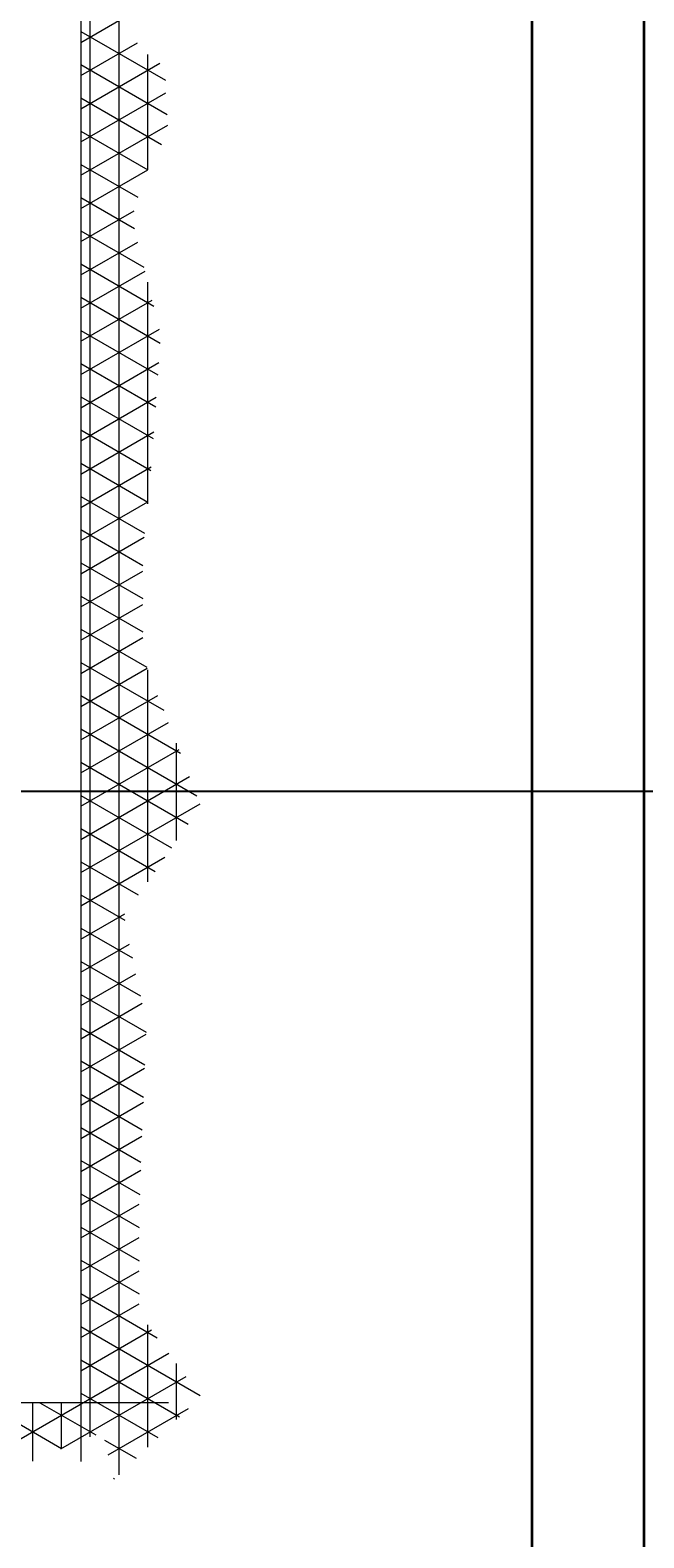
# Model space of a CAD drawing. Units: inches. Extents: x 3731 to 4318, y 1310 to 2388.
# Tile 54 of 57: x 4212 to 4239, y 2229 to 2296. Entities that reach past the tile are written whole.
import ezdxf

# ---------------------------------------------------------------- set-up
doc = ezdxf.new("R2010")
doc.units = ezdxf.units.IN
for name, color, linetype, lineweight in [('A-ANNO-DIMS', 2, 'Continuous', 18), ('A-FURN', 8, 'Continuous', 13), ('A-WALL', 7, 'Continuous', 35)]:
    doc.layers.add(name, color=color, linetype=linetype, lineweight=lineweight)
doc.styles.get("Standard").update_dxf_attribs({"font": 'arial.ttf'})
doc.dimstyles.get("Standard").update_dxf_attribs({"dimtxt": 0.18, "dimasz": 0.18, "dimexe": 0.18, "dimexo": 0.0625, "dimgap": 0.09, "dimtad": 0, "dimtih": 1, "dimtoh": 1, "dimdec": 4, "dimzin": 0, "dimdsep": 46, "dimtxsty": 'Standard', "dimcen": 0.09, "dimadec": 0, "dimazin": 0, "dimtfac": 1, "dimtdec": 4, "dimtofl": 0, "dimtmove": 0, "dimatfit": 3, "dimfxl": 1, "dimtolj": 1, "dimtzin": 0, "dimarcsym": 0})

# ---------------------------------------------------------------- blocks, each defined once
blk = doc.blocks.new('A$C200C7901')
for p, q in [((2.3121, 1.6596), (2.3121, 0.0201)), ((2.4073, 0.0839), (0.9625, 0.0839))]:
    blk.add_line(p, q)
at = {"linetype": 'ByBlock'}
for p, q in [((2.3224, 0.0468), (2.3224, 1.6627)), ((2.3224, 0.0468), (2.3224, 1.6627)), ((2.3537, 0.0056), (2.3537, 1.634)), ((2.3537, 0.0056), (2.3537, 1.634)), ((2.3121, 1.5619), (2.3654, 1.5926)), ((2.3121, 1.5619), (2.3654, 1.5926)), ((2.3121, 1.5738), (2.404, 1.5208)), ((2.3121, 1.5738), (2.404, 1.5208)), ((2.3121, 1.5258), (2.3739, 1.5615)), ((2.3121, 1.5258), (2.3739, 1.5615)), ((2.3849, 1.4236), (2.3849, 1.5486)), ((2.3849, 1.4236), (2.3849, 1.5486)), ((2.3121, 1.4897), (2.3979, 1.5393)), ((2.3121, 1.4897), (2.3979, 1.5393)), ((2.3121, 1.5377), (2.406, 1.4835)), ((2.3121, 1.5377), (2.406, 1.4835)), ((2.3121, 1.4537), (2.4047, 1.5071)), ((2.3121, 1.4537), (2.4047, 1.5071)), ((2.3121, 1.5016), (2.3997, 1.4511)), ((2.3121, 1.5016), (2.3997, 1.4511)), ((2.3121, 1.4176), (2.4067, 1.4721)), ((2.3121, 1.4176), (2.4067, 1.4721)), ((2.3121, 1.4655), (2.3849, 1.4235)), ((2.3121, 1.4655), (2.3849, 1.4235)), ((2.3121, 1.4294), (2.3741, 1.3937)), ((2.3121, 1.4294), (2.3741, 1.3937)), ((2.3121, 1.3815), (2.3848, 1.4235)), ((2.3121, 1.3815), (2.3848, 1.4235)), ((2.3121, 1.3934), (2.3703, 1.3598)), ((2.3121, 1.3934), (2.3703, 1.3598)), ((2.3121, 1.3454), (2.37, 1.3788)), ((2.3121, 1.3454), (2.37, 1.3788)), ((2.3121, 1.3573), (2.3808, 1.3176)), ((2.3121, 1.3573), (2.3808, 1.3176)), ((2.3121, 1.3093), (2.374, 1.345)), ((2.3121, 1.3093), (2.374, 1.345)), ((2.3121, 1.3212), (2.3914, 1.2754)), ((2.3121, 1.3212), (2.3914, 1.2754)), ((2.3121, 1.2732), (2.3819, 1.3135)), ((2.3121, 1.2732), (2.3819, 1.3135)), ((2.3849, 1.0607), (2.3849, 1.3013)), ((2.3849, 1.0607), (2.3849, 1.3013)), ((2.3121, 1.2851), (2.3985, 1.2352)), ((2.3121, 1.2851), (2.3985, 1.2352)), ((2.3121, 1.2371), (2.3898, 1.282)), ((2.3121, 1.2371), (2.3898, 1.282)), ((2.3121, 1.2011), (2.3976, 1.2504)), ((2.3121, 1.2011), (2.3976, 1.2504)), ((2.3121, 1.249), (2.396, 1.2006)), ((2.3121, 1.249), (2.396, 1.2006)), ((2.3121, 1.165), (2.397, 1.214)), ((2.3121, 1.165), (2.397, 1.214)), ((2.3121, 1.2129), (2.3935, 1.166)), ((2.3121, 1.2129), (2.3935, 1.166)), ((2.3121, 1.1768), (2.3909, 1.1314)), ((2.3121, 1.1768), (2.3909, 1.1314)), ((2.3121, 1.1289), (2.3942, 1.1763)), ((2.3121, 1.1289), (2.3942, 1.1763)), ((2.3121, 1.1408), (2.3884, 1.0967)), ((2.3121, 1.1408), (2.3884, 1.0967)), ((2.3121, 1.0928), (2.3915, 1.1386)), ((2.3121, 1.0928), (2.3915, 1.1386)), ((2.3121, 1.1047), (2.3851, 1.0625)), ((2.3121, 1.1047), (2.3851, 1.0625)), ((2.3121, 1.0567), (2.3887, 1.1009)), ((2.3121, 1.0567), (2.3887, 1.1009)), ((2.3121, 1.0686), (2.3813, 1.0286)), ((2.3121, 1.0686), (2.3813, 1.0286)), ((2.3121, 1.0206), (2.3851, 1.0628)), ((2.3121, 1.0206), (2.3851, 1.0628)), ((2.3121, 1.0325), (2.3795, 0.9936)), ((2.3121, 1.0325), (2.3795, 0.9936)), ((2.3121, 0.9846), (2.3809, 1.0242)), ((2.3121, 0.9846), (2.3809, 1.0242)), ((2.3121, 0.9964), (2.3795, 0.9575)), ((2.3121, 0.9964), (2.3795, 0.9575)), ((2.3121, 0.9485), (2.3795, 0.9874)), ((2.3121, 0.9485), (2.3795, 0.9874)), ((2.3121, 0.9603), (2.3795, 0.9215)), ((2.3121, 0.9603), (2.3795, 0.9215)), ((2.3121, 0.9124), (2.3795, 0.9513)), ((2.3121, 0.9124), (2.3795, 0.9513)), ((2.3121, 0.9243), (2.3838, 0.8829)), ((2.3121, 0.9243), (2.3838, 0.8829)), ((2.3121, 0.8763), (2.3795, 0.9152)), ((2.3121, 0.8763), (2.3795, 0.9152)), ((2.3121, 0.8882), (2.4022, 0.8362)), ((2.3121, 0.8882), (2.4022, 0.8362)), ((2.3121, 0.8402), (2.3842, 0.8818)), ((2.3121, 0.8402), (2.3842, 0.8818)), ((2.3849, 0.6497), (2.3849, 0.8801)), ((2.3849, 0.6497), (2.3849, 0.8801)), ((2.3121, 0.8041), (2.3958, 0.8524)), ((2.3121, 0.8041), (2.3958, 0.8524)), ((2.3121, 0.8521), (2.4205, 0.7895)), ((2.3121, 0.8521), (2.4205, 0.7895)), ((2.3121, 0.7681), (2.4073, 0.823)), ((2.3121, 0.7681), (2.4073, 0.823)), ((2.3121, 0.816), (2.4384, 0.7431)), ((2.3121, 0.816), (2.4384, 0.7431)), ((2.3121, 0.732), (2.4189, 0.7936)), ((2.3121, 0.732), (2.4189, 0.7936)), ((2.4162, 0.6946), (2.4162, 0.8006)), ((2.4162, 0.6946), (2.4162, 0.8006)), ((2.3121, 0.7799), (2.4287, 0.7126)), ((2.3121, 0.7799), (2.4287, 0.7126)), ((2.3121, 0.6959), (2.4303, 0.7641)), ((2.3121, 0.6959), (2.4303, 0.7641)), ((2.3121, 0.7438), (2.4108, 0.6869)), ((2.3121, 0.7438), (2.4108, 0.6869)), ((2.3121, 0.6598), (2.4417, 0.7346)), ((2.3121, 0.6598), (2.4417, 0.7346)), ((2.3121, 0.7078), (2.3929, 0.6611)), ((2.3121, 0.7078), (2.3929, 0.6611)), ((2.3121, 0.6237), (2.4036, 0.6765)), ((2.3121, 0.6237), (2.4036, 0.6765)), ((2.3121, 0.6717), (2.3744, 0.6357)), ((2.3121, 0.6717), (2.3744, 0.6357)), ((2.3121, 0.6356), (2.3598, 0.6081)), ((2.3121, 0.6356), (2.3598, 0.6081)), ((2.3121, 0.5876), (2.3598, 0.6151)), ((2.3121, 0.5876), (2.3598, 0.6151)), ((2.3121, 0.5995), (2.3682, 0.5671)), ((2.3121, 0.5995), (2.3682, 0.5671)), ((2.3121, 0.5515), (2.365, 0.5821)), ((2.3121, 0.5515), (2.365, 0.5821)), ((2.3121, 0.5634), (2.3771, 0.5259)), ((2.3121, 0.5634), (2.3771, 0.5259)), ((2.3121, 0.5155), (2.3719, 0.55)), ((2.3121, 0.5155), (2.3719, 0.55)), ((2.3121, 0.5273), (2.383, 0.4864)), ((2.3121, 0.5273), (2.383, 0.4864)), ((2.3121, 0.4794), (2.3788, 0.5179)), ((2.3121, 0.4794), (2.3788, 0.5179)), ((2.3121, 0.4912), (2.3817, 0.4511)), ((2.3121, 0.4912), (2.3817, 0.4511)), ((2.3121, 0.4433), (2.383, 0.4842)), ((2.3121, 0.4433), (2.383, 0.4842)), ((2.3121, 0.4552), (2.3803, 0.4158)), ((2.3121, 0.4552), (2.3803, 0.4158)), ((2.3121, 0.4072), (2.3815, 0.4473)), ((2.3121, 0.4072), (2.3815, 0.4473)), ((2.3121, 0.4191), (2.3789, 0.3805)), ((2.3121, 0.4191), (2.3789, 0.3805)), ((2.3121, 0.3711), (2.3801, 0.4103)), ((2.3121, 0.3711), (2.3801, 0.4103)), ((2.3121, 0.383), (2.3775, 0.3452)), ((2.3121, 0.383), (2.3775, 0.3452)), ((2.3121, 0.335), (2.3786, 0.3734)), ((2.3121, 0.335), (2.3786, 0.3734)), ((2.3121, 0.3469), (2.3761, 0.31)), ((2.3121, 0.3469), (2.3761, 0.31)), ((2.3121, 0.299), (2.3772, 0.3365)), ((2.3121, 0.299), (2.3772, 0.3365)), ((2.3121, 0.3108), (2.3755, 0.2742)), ((2.3121, 0.3108), (2.3755, 0.2742)), ((2.3121, 0.2629), (2.3757, 0.2996)), ((2.3121, 0.2629), (2.3757, 0.2996)), ((2.3121, 0.2747), (2.3755, 0.2381)), ((2.3121, 0.2747), (2.3755, 0.2381)), ((2.3121, 0.2268), (2.3755, 0.2634)), ((2.3121, 0.2268), (2.3755, 0.2634)), ((2.3121, 0.2387), (2.3755, 0.202)), ((2.3121, 0.2387), (2.3755, 0.202)), ((2.3121, 0.1907), (2.3755, 0.2273)), ((2.3121, 0.1907), (2.3755, 0.2273)), ((2.3121, 0.2026), (2.3953, 0.1545)), ((2.3121, 0.2026), (2.3953, 0.1545)), ((2.3121, 0.1546), (2.3755, 0.1912)), ((2.3121, 0.1546), (2.3755, 0.1912)), ((2.3121, 0.1665), (2.4419, 0.0916)), ((2.3121, 0.1665), (2.4419, 0.0916)), ((2.3849, 0.0355), (2.3849, 0.1686)), ((2.3849, 0.0355), (2.3849, 0.1686)), ((2.3121, 0.1185), (2.3891, 0.163)), ((2.3121, 0.1185), (2.3891, 0.163)), ((2.2208, 0.0297), (2.4078, 0.1377)), ((2.2208, 0.0297), (2.4078, 0.1377)), ((2.3121, 0.1304), (2.4193, 0.0685)), ((2.3121, 0.1304), (2.4193, 0.0685)), ((2.4162, 0.0655), (2.4162, 0.1264)), ((2.4162, 0.0655), (2.4162, 0.1264)), ((2.2903, 0.0337), (2.4265, 0.1124)), ((2.2903, 0.0337), (2.4265, 0.1124)), ((2.2051, 0.0839), (2.2913, 0.0342)), ((2.2051, 0.0839), (2.2913, 0.0342)), ((2.2599, 0.0205), (2.2599, 0.0839)), ((2.2599, 0.0205), (2.2599, 0.0839)), ((2.2676, 0.0839), (2.3285, 0.0488)), ((2.2676, 0.0839), (2.3285, 0.0488)), ((2.2912, 0.0341), (2.2912, 0.0839)), ((2.2912, 0.0341), (2.2912, 0.0839)), ((2.3121, 0.0943), (2.3958, 0.046)), ((2.3121, 0.0943), (2.3958, 0.046)), ((2.3417, 0.0273), (2.429, 0.0777)), ((2.3417, 0.0273), (2.429, 0.0777)), ((2.338, 0.0433), (2.3723, 0.0235)), ((2.338, 0.0433), (2.3723, 0.0235)), ((2.3476, 0.0017), (2.3488, 0.001)), ((2.3476, 0.0017), (2.3488, 0.001))]:
    blk.add_line(p, q, dxfattribs=at)
blk = doc.blocks.new('*D37')
at = {"layer": 'A-ANNO-DIMS', "color": 0, "lineweight": -2, "transparency": 16777216}
for p, q in [((4239.271, 2338.382), (4318.341, 2338.382)), ((4318.161, 2338.202), (4318.161, 2300.563)), ((4318.161, 2262.562), (4318.161, 2300.2)), ((4103.271, 2262.382), (4318.341, 2262.382))]:
    blk.add_line(p, q, dxfattribs=at)
at = {"layer": 'A-ANNO-DIMS', "color": 0, "transparency": 16777216}
for points in [[(4318.131, 2338.202), (4318.191, 2338.202), (4318.161, 2338.382)], [(4318.131, 2262.562), (4318.191, 2262.562), (4318.161, 2262.382)]]:
    blk.add_solid(points, dxfattribs=at)
at = {"layer": 'Defpoints', "color": 0, "transparency": 16777216}
for p in [(4239.209, 2338.382), (4318.161, 2338.382), (4103.209, 2262.382)]:
    blk.add_point(p, dxfattribs=at)
at = {"layer": 'A-ANNO-DIMS', "color": 0, "transparency": 16777216, "insert": (4318.161, 2300.382), "char_height": 0.18, "attachment_point": 5}
blk.add_mtext('\\A1;76', dxfattribs=at)
blk = doc.blocks.new('*D38')
at = {"layer": 'A-ANNO-DIMS', "color": 0, "lineweight": -2, "transparency": 16777216}
for p, q in [((4103.271, 2262.382), (4318.341, 2262.382)), ((4318.161, 2262.202), (4318.161, 2103.064)), ((4318.161, 1943.562), (4318.161, 2102.7)), ((4234.271, 1943.382), (4318.341, 1943.382))]:
    blk.add_line(p, q, dxfattribs=at)
at = {"layer": 'A-ANNO-DIMS', "color": 0, "transparency": 16777216}
for points in [[(4318.131, 2262.202), (4318.191, 2262.202), (4318.161, 2262.382)], [(4318.131, 1943.562), (4318.191, 1943.562), (4318.161, 1943.382)]]:
    blk.add_solid(points, dxfattribs=at)
at = {"layer": 'Defpoints', "color": 0, "transparency": 16777216}
for p in [(4103.209, 2262.382), (4318.161, 2262.382), (4234.209, 1943.382)]:
    blk.add_point(p, dxfattribs=at)
at = {"layer": 'A-ANNO-DIMS', "color": 0, "transparency": 16777216, "insert": (4318.161, 2102.882), "char_height": 0.18, "attachment_point": 5}
blk.add_mtext('\\A1;319', dxfattribs=at)

msp = doc.modelspace()

# ---------------------------------------------------------------- linework, layer by layer
at = {"layer": 'A-WALL'}
for p, q in [((4239.209, 2338.382), (4239.209, 1708.382)), ((4234.209, 2333.382), (4234.209, 2189.382))]:
    msp.add_line(p, q, dxfattribs=at)

# ---------------------------------------------------------------- block references
at = {"layer": 'A-FURN', "xscale": 41.1071563136412, "yscale": 41.1071563136412, "zscale": 41.1071563136412}
msp.add_blockref('A$C200C7901', (4119.004, 2231.625), dxfattribs=at)

# ---------------------------------------------------------------- dimensions: what is measured, and where the dimension line sits
at = {"layer": 'A-ANNO-DIMS'}
for base, p1, p2, picture, middle in [((4318.161, 2338.382), (4103.209, 2262.382), (4239.209, 2338.382), '*D37', (4318.161, 2300.382)), ((4318.161, 2262.382), (4234.209, 1943.382), (4103.209, 2262.382), '*D38', (4318.161, 2102.882))]:
    dim = msp.add_linear_dim(base=base, p1=p1, p2=p2, angle=90, dimstyle='Standard', override={"dimdec": 0, "dimlfac": 1, "dimrnd": 0, "dimzin": 0, "dimdsep": 46, "dimlunit": 2}, dxfattribs=at)
    dim.commit()
    dim.dimension.update_dxf_attribs({"geometry": picture, "text_midpoint": middle})

doc.saveas('drawing.dxf')
